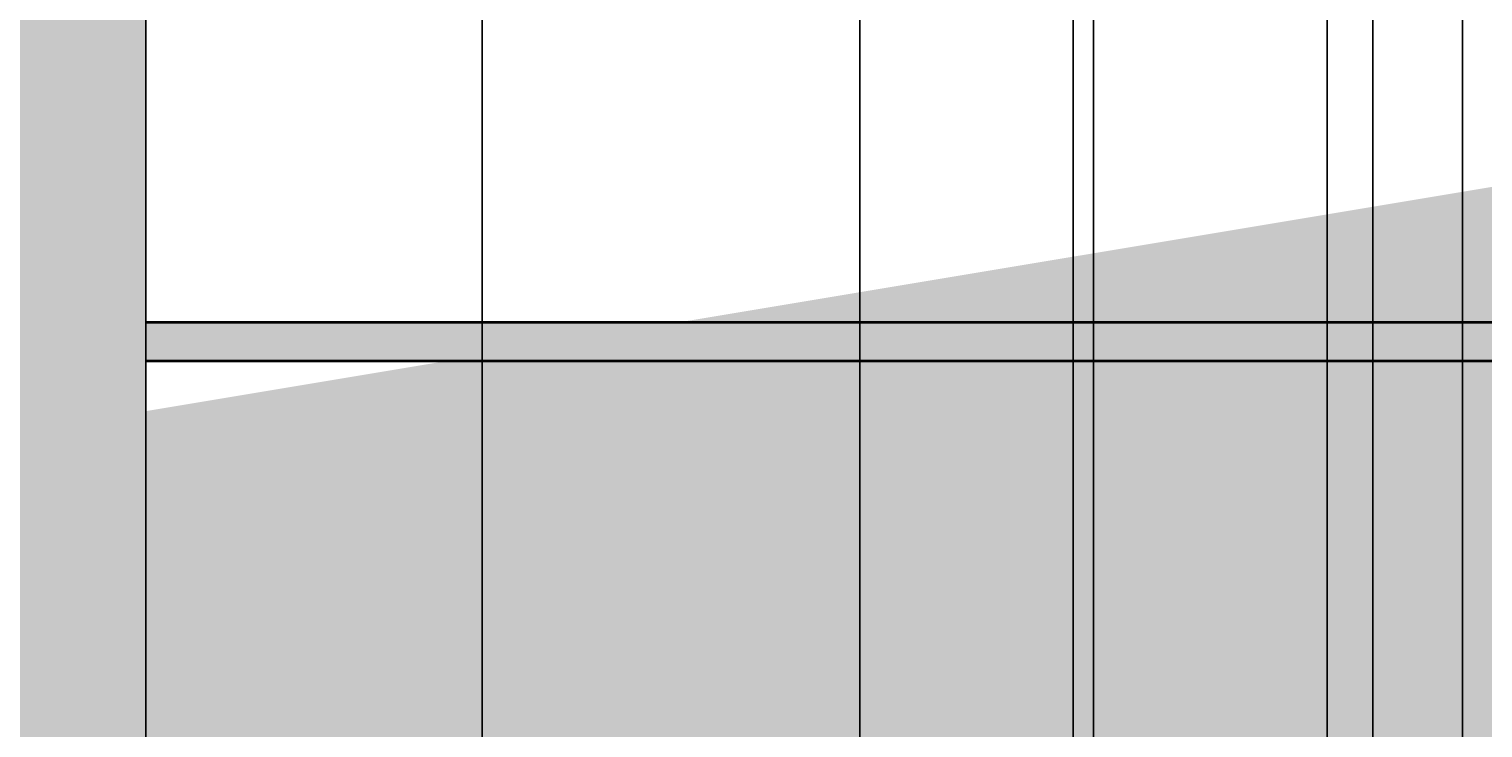
# Model space of a CAD drawing. Units: millimetres. Extents: x -22994 to 29398, y -19990 to 20176.
# Tile 43 of 135: x 99 to 136, y 78 to 96. Entities that reach past the tile are written whole.
import ezdxf

# ---------------------------------------------------------------- set-up
doc = ezdxf.new("R2010")
doc.units = ezdxf.units.MM
doc.header["$MEASUREMENT"] = 0
for name, color, linetype, lineweight in [('M-DIMS', 2, 'Continuous', 18), ('M-EQPM', 7, 'Continuous', 25), ('M-EQPM-PATT', 7, 'Continuous', 18), ('M-PIPE', 7, 'Continuous', 35)]:
    doc.layers.add(name, color=color, linetype=linetype, lineweight=lineweight)
doc.styles.get("Standard").update_dxf_attribs({"font": 'arial.ttf'})
doc.dimstyles.get("Standard").update_dxf_attribs({"dimtxt": 0.18, "dimasz": 10000, "dimexe": 0.18, "dimexo": 0.0625, "dimgap": 0.09, "dimtad": 0, "dimtih": 1, "dimtoh": 1, "dimdec": 0, "dimzin": 0, "dimdsep": 46, "dimtxsty": 'Standard', "dimcen": 0.09, "dimadec": 0, "dimazin": 0, "dimtfac": 1, "dimtdec": 0, "dimtofl": 0, "dimtmove": 0, "dimatfit": 3, "dimfxl": 1, "dimtolj": 1, "dimtzin": 0, "dimlwd": 30, "dimarcsym": 0})

# ---------------------------------------------------------------- blocks, each defined once
blk = doc.blocks.new('*D2')
at = {"layer": 'Defpoints', "color": 0, "transparency": 16777216}
for p in [(6.677, 10.271), (290.852, 10.271), (290.852, -5.079)]:
    blk.add_point(p, dxfattribs=at)
at = {"layer": 'M-DIMS', "color": 0, "lineweight": -2, "transparency": 16777216}
for p, q in [((6.677, 10.209), (6.677, -5.259)), ((290.852, 10.209), (290.852, -5.259))]:
    blk.add_line(p, q, dxfattribs=at)
at = {"layer": 'M-DIMS', "color": 0, "lineweight": 30, "transparency": 16777216}
for p, q in [((-9993.323, -5.079), (-19993.323, -5.079)), ((10290.852, -5.079), (20290.852, -5.079))]:
    blk.add_line(p, q, dxfattribs=at)
at = {"layer": 'M-DIMS', "color": 0, "transparency": 16777216}
for points in [[(-9993.323, 1661.588), (-9993.323, -1671.745), (6.677, -5.079)], [(10290.852, 1661.588), (10290.852, -1671.745), (290.852, -5.079)]]:
    blk.add_solid(points, dxfattribs=at)
at = {"layer": 'M-DIMS', "color": 0, "transparency": 16777216, "insert": (148.765, -5.079), "char_height": 0.18, "attachment_point": 5}
blk.add_mtext('\\A1;284.2', dxfattribs=at)
blk = doc.blocks.new('*D3')
at = {"layer": 'Defpoints', "color": 0, "transparency": 16777216}
for p in [(110.265, 204.165), (110.265, 176.366), (95.833, 127.967)]:
    blk.add_point(p, dxfattribs=at)
at = {"layer": 'M-DIMS', "color": 0, "lineweight": -2, "transparency": 16777216}
for p, q in [((95.833, 128.03), (95.833, 204.345)), ((110.265, 176.429), (110.265, 204.345))]:
    blk.add_line(p, q, dxfattribs=at)
at = {"layer": 'M-DIMS', "color": 0, "lineweight": 30, "transparency": 16777216}
for p, q in [((-9904.167, 204.165), (-19904.167, 204.165)), ((10110.265, 204.165), (20110.265, 204.165))]:
    blk.add_line(p, q, dxfattribs=at)
at = {"layer": 'M-DIMS', "color": 0, "transparency": 16777216}
for points in [[(-9904.167, 1870.832), (-9904.167, -1462.501), (95.833, 204.165)], [(10110.265, 1870.832), (10110.265, -1462.501), (110.265, 204.165)]]:
    blk.add_solid(points, dxfattribs=at)
at = {"layer": 'M-DIMS', "color": 0, "transparency": 16777216, "insert": (103.049, 204.165), "char_height": 0.18, "attachment_point": 5}
blk.add_mtext('\\A1;14.432', dxfattribs=at)
blk = doc.blocks.new('*D4')
at = {"layer": 'Defpoints', "color": 0, "transparency": 16777216}
for p in [(116.265, 204.165), (110.265, 176.366), (116.265, 176.366)]:
    blk.add_point(p, dxfattribs=at)
at = {"layer": 'M-DIMS', "color": 0, "lineweight": -2, "transparency": 16777216}
for p, q in [((110.265, 176.429), (110.265, 204.345)), ((116.265, 176.429), (116.265, 204.345))]:
    blk.add_line(p, q, dxfattribs=at)
at = {"layer": 'M-DIMS', "color": 0, "lineweight": 30, "transparency": 16777216}
for p, q in [((-9889.735, 204.165), (-19889.735, 204.165)), ((10116.265, 204.165), (20116.265, 204.165))]:
    blk.add_line(p, q, dxfattribs=at)
at = {"layer": 'M-DIMS', "color": 0, "transparency": 16777216}
for points in [[(-9889.735, 1870.832), (-9889.735, -1462.501), (110.265, 204.165)], [(10116.265, 1870.832), (10116.265, -1462.501), (116.265, 204.165)]]:
    blk.add_solid(points, dxfattribs=at)
at = {"layer": 'M-DIMS', "color": 0, "transparency": 16777216, "insert": (113.265, 204.165), "char_height": 0.18, "attachment_point": 5}
blk.add_mtext('\\A1;6', dxfattribs=at)
blk = doc.blocks.new('*D5')
at = {"layer": 'Defpoints', "color": 0, "transparency": 16777216}
for p in [(181.265, 204.165), (116.265, 176.366), (181.265, 176.366)]:
    blk.add_point(p, dxfattribs=at)
at = {"layer": 'M-DIMS', "color": 0, "lineweight": -2, "transparency": 16777216}
for p, q in [((116.265, 176.429), (116.265, 204.345)), ((181.265, 176.429), (181.265, 204.345))]:
    blk.add_line(p, q, dxfattribs=at)
at = {"layer": 'M-DIMS', "color": 0, "lineweight": 30, "transparency": 16777216}
for p, q in [((-9883.735, 204.165), (-19883.735, 204.165)), ((10181.265, 204.165), (20181.265, 204.165))]:
    blk.add_line(p, q, dxfattribs=at)
at = {"layer": 'M-DIMS', "color": 0, "transparency": 16777216}
for points in [[(-9883.735, 1870.832), (-9883.735, -1462.501), (116.265, 204.165)], [(10181.265, 1870.832), (10181.265, -1462.501), (181.265, 204.165)]]:
    blk.add_solid(points, dxfattribs=at)
at = {"layer": 'M-DIMS', "color": 0, "transparency": 16777216, "insert": (148.765, 204.165), "char_height": 0.18, "attachment_point": 5}
blk.add_mtext('\\A1;65', dxfattribs=at)
blk = doc.blocks.new('*D6')
at = {"layer": 'Defpoints', "color": 0, "transparency": 16777216}
for p in [(187.265, 204.165), (181.265, 176.366), (187.265, 176.366)]:
    blk.add_point(p, dxfattribs=at)
at = {"layer": 'M-DIMS', "color": 0, "lineweight": -2, "transparency": 16777216}
for p, q in [((181.265, 176.429), (181.265, 204.345)), ((187.265, 176.429), (187.265, 204.345))]:
    blk.add_line(p, q, dxfattribs=at)
at = {"layer": 'M-DIMS', "color": 0, "lineweight": 30, "transparency": 16777216}
for p, q in [((-9818.735, 204.165), (-19818.735, 204.165)), ((10187.265, 204.165), (20187.265, 204.165))]:
    blk.add_line(p, q, dxfattribs=at)
at = {"layer": 'M-DIMS', "color": 0, "transparency": 16777216}
for points in [[(-9818.735, 1870.832), (-9818.735, -1462.501), (181.265, 204.165)], [(10187.265, 1870.832), (10187.265, -1462.501), (187.265, 204.165)]]:
    blk.add_solid(points, dxfattribs=at)
at = {"layer": 'M-DIMS', "color": 0, "transparency": 16777216, "insert": (184.265, 204.165), "char_height": 0.18, "attachment_point": 5}
blk.add_mtext('\\A1;6', dxfattribs=at)
blk = doc.blocks.new('*D7')
at = {"layer": 'Defpoints', "color": 0, "transparency": 16777216}
for p in [(201.697, 204.165), (187.265, 176.366), (201.697, 127.967)]:
    blk.add_point(p, dxfattribs=at)
at = {"layer": 'M-DIMS', "color": 0, "lineweight": -2, "transparency": 16777216}
for p, q in [((187.265, 176.429), (187.265, 204.345)), ((201.697, 128.03), (201.697, 204.345))]:
    blk.add_line(p, q, dxfattribs=at)
at = {"layer": 'M-DIMS', "color": 0, "lineweight": 30, "transparency": 16777216}
for p, q in [((-9812.735, 204.165), (-19812.735, 204.165)), ((10201.697, 204.165), (20201.697, 204.165))]:
    blk.add_line(p, q, dxfattribs=at)
at = {"layer": 'M-DIMS', "color": 0, "transparency": 16777216}
for points in [[(-9812.735, 1870.832), (-9812.735, -1462.501), (187.265, 204.165)], [(10201.697, 1870.832), (10201.697, -1462.501), (201.697, 204.165)]]:
    blk.add_solid(points, dxfattribs=at)
at = {"layer": 'M-DIMS', "color": 0, "transparency": 16777216, "insert": (194.481, 204.165), "char_height": 0.18, "attachment_point": 5}
blk.add_mtext('\\A1;14.432', dxfattribs=at)
blk = doc.blocks.new('*D8')
at = {"layer": 'Defpoints', "color": 0, "transparency": 16777216}
for p in [(227.648, 204.165), (227.648, 146.73), (201.697, 127.967)]:
    blk.add_point(p, dxfattribs=at)
at = {"layer": 'M-DIMS', "color": 0, "lineweight": -2, "transparency": 16777216}
for p, q in [((201.697, 128.03), (201.697, 204.345)), ((227.648, 146.792), (227.648, 204.345))]:
    blk.add_line(p, q, dxfattribs=at)
at = {"layer": 'M-DIMS', "color": 0, "lineweight": 30, "transparency": 16777216}
for p, q in [((-9798.303, 204.165), (-19798.303, 204.165)), ((10227.648, 204.165), (20227.648, 204.165))]:
    blk.add_line(p, q, dxfattribs=at)
at = {"layer": 'M-DIMS', "color": 0, "transparency": 16777216}
for points in [[(-9798.303, 1870.832), (-9798.303, -1462.501), (201.697, 204.165)], [(10227.648, 1870.832), (10227.648, -1462.501), (227.648, 204.165)]]:
    blk.add_solid(points, dxfattribs=at)
at = {"layer": 'M-DIMS', "color": 0, "transparency": 16777216, "insert": (214.673, 204.165), "char_height": 0.18, "attachment_point": 5}
blk.add_mtext('\\A1;25.95', dxfattribs=at)
blk = doc.blocks.new('*D9')
at = {"layer": 'Defpoints', "color": 0, "transparency": 16777216}
for p in [(187.265, 176.366), (306.202, 176.366), (290.852, 10.271)]:
    blk.add_point(p, dxfattribs=at)
at = {"layer": 'M-DIMS', "color": 0, "lineweight": 30, "transparency": 16777216}
for p, q in [((306.202, 10176.366), (306.202, 20176.366)), ((306.202, -9989.729), (306.202, -19989.729))]:
    blk.add_line(p, q, dxfattribs=at)
at = {"layer": 'M-DIMS', "color": 0, "lineweight": -2, "transparency": 16777216}
for p, q in [((187.327, 176.366), (306.382, 176.366)), ((290.915, 10.271), (306.382, 10.271))]:
    blk.add_line(p, q, dxfattribs=at)
at = {"layer": 'M-DIMS', "color": 0, "transparency": 16777216}
for points in [[(-1360.465, 10176.366), (1972.869, 10176.366), (306.202, 176.366)], [(-1360.465, -9989.729), (1972.869, -9989.729), (306.202, 10.271)]]:
    blk.add_solid(points, dxfattribs=at)
at = {"layer": 'M-DIMS', "color": 0, "transparency": 16777216, "insert": (306.202, 93.319), "char_height": 0.18, "attachment_point": 5}
blk.add_mtext('\\A1;166.1', dxfattribs=at)
blk = doc.blocks.new('*D10')
at = {"layer": 'Defpoints', "color": 0, "transparency": 16777216}
for p in [(125.65, 136.071), (133.346, 136.071), (133.346, -5.079)]:
    blk.add_point(p, dxfattribs=at)
at = {"layer": 'M-DIMS', "color": 0, "lineweight": -2, "transparency": 16777216}
for p, q in [((125.65, 136.009), (125.65, -5.259)), ((133.346, 136.009), (133.346, -5.259))]:
    blk.add_line(p, q, dxfattribs=at)
at = {"layer": 'M-DIMS', "color": 0, "lineweight": 30, "transparency": 16777216}
for p, q in [((-9874.35, -5.079), (-19874.35, -5.079)), ((10133.346, -5.079), (20133.346, -5.079))]:
    blk.add_line(p, q, dxfattribs=at)
at = {"layer": 'M-DIMS', "color": 0, "transparency": 16777216}
for points in [[(-9874.35, 1661.588), (-9874.35, -1671.745), (125.65, -5.079)], [(10133.346, 1661.588), (10133.346, -1671.745), (133.346, -5.079)]]:
    blk.add_solid(points, dxfattribs=at)
at = {"layer": 'M-DIMS', "color": 0, "transparency": 16777216, "insert": (129.498, -5.079), "char_height": 0.18, "attachment_point": 5}
blk.add_mtext('\\A1;7.696', dxfattribs=at)
blk = doc.blocks.new('*D11')
at = {"layer": 'Defpoints', "color": 0, "transparency": 16777216}
for p in [(133.346, 136.071), (135.65, 136.071), (135.65, -5.079)]:
    blk.add_point(p, dxfattribs=at)
at = {"layer": 'M-DIMS', "color": 0, "lineweight": -2, "transparency": 16777216}
for p, q in [((133.346, 136.009), (133.346, -5.259)), ((135.65, 136.009), (135.65, -5.259))]:
    blk.add_line(p, q, dxfattribs=at)
at = {"layer": 'M-DIMS', "color": 0, "lineweight": 30, "transparency": 16777216}
for p, q in [((-9866.654, -5.079), (-19866.654, -5.079)), ((10135.65, -5.079), (20135.65, -5.079))]:
    blk.add_line(p, q, dxfattribs=at)
at = {"layer": 'M-DIMS', "color": 0, "transparency": 16777216}
for points in [[(-9866.654, 1661.588), (-9866.654, -1671.745), (133.346, -5.079)], [(10135.65, 1661.588), (10135.65, -1671.745), (135.65, -5.079)]]:
    blk.add_solid(points, dxfattribs=at)
at = {"layer": 'M-DIMS', "color": 0, "transparency": 16777216, "insert": (134.498, -5.079), "char_height": 0.18, "attachment_point": 5}
blk.add_mtext('\\A1;2.304', dxfattribs=at)
blk = doc.blocks.new('*D12')
at = {"layer": 'Defpoints', "color": 0, "transparency": 16777216}
for p in [(135.65, 136.071), (145.65, 136.071), (145.65, -5.079)]:
    blk.add_point(p, dxfattribs=at)
at = {"layer": 'M-DIMS', "color": 0, "lineweight": -2, "transparency": 16777216}
for p, q in [((135.65, 136.009), (135.65, -5.259)), ((145.65, 136.009), (145.65, -5.259))]:
    blk.add_line(p, q, dxfattribs=at)
at = {"layer": 'M-DIMS', "color": 0, "lineweight": 30, "transparency": 16777216}
for p, q in [((-9864.35, -5.079), (-19864.35, -5.079)), ((10145.65, -5.079), (20145.65, -5.079))]:
    blk.add_line(p, q, dxfattribs=at)
at = {"layer": 'M-DIMS', "color": 0, "transparency": 16777216}
for points in [[(-9864.35, 1661.588), (-9864.35, -1671.745), (135.65, -5.079)], [(10145.65, 1661.588), (10145.65, -1671.745), (145.65, -5.079)]]:
    blk.add_solid(points, dxfattribs=at)
at = {"layer": 'M-DIMS', "color": 0, "transparency": 16777216, "insert": (140.65, -5.079), "char_height": 0.18, "attachment_point": 5}
blk.add_mtext('\\A1;10', dxfattribs=at)
blk = doc.blocks.new('*D13')
at = {"layer": 'Defpoints', "color": 0, "transparency": 16777216}
for p in [(145.65, 136.071), (155.65, 136.071), (155.65, -5.079)]:
    blk.add_point(p, dxfattribs=at)
at = {"layer": 'M-DIMS', "color": 0, "lineweight": -2, "transparency": 16777216}
for p, q in [((145.65, 136.009), (145.65, -5.259)), ((155.65, 136.009), (155.65, -5.259))]:
    blk.add_line(p, q, dxfattribs=at)
at = {"layer": 'M-DIMS', "color": 0, "lineweight": 30, "transparency": 16777216}
for p, q in [((-9854.35, -5.079), (-19854.35, -5.079)), ((10155.65, -5.079), (20155.65, -5.079))]:
    blk.add_line(p, q, dxfattribs=at)
at = {"layer": 'M-DIMS', "color": 0, "transparency": 16777216}
for points in [[(-9854.35, 1661.588), (-9854.35, -1671.745), (145.65, -5.079)], [(10155.65, 1661.588), (10155.65, -1671.745), (155.65, -5.079)]]:
    blk.add_solid(points, dxfattribs=at)
at = {"layer": 'M-DIMS', "color": 0, "transparency": 16777216, "insert": (150.65, -5.079), "char_height": 0.18, "attachment_point": 5}
blk.add_mtext('\\A1;10', dxfattribs=at)
blk = doc.blocks.new('*D14')
at = {"layer": 'Defpoints', "color": 0, "transparency": 16777216}
for p in [(155.65, 136.071), (165.65, 136.071), (165.65, -5.079)]:
    blk.add_point(p, dxfattribs=at)
at = {"layer": 'M-DIMS', "color": 0, "lineweight": -2, "transparency": 16777216}
for p, q in [((155.65, 136.009), (155.65, -5.259)), ((165.65, 136.009), (165.65, -5.259))]:
    blk.add_line(p, q, dxfattribs=at)
at = {"layer": 'M-DIMS', "color": 0, "lineweight": 30, "transparency": 16777216}
for p, q in [((-9844.35, -5.079), (-19844.35, -5.079)), ((10165.65, -5.079), (20165.65, -5.079))]:
    blk.add_line(p, q, dxfattribs=at)
at = {"layer": 'M-DIMS', "color": 0, "transparency": 16777216}
for points in [[(-9844.35, 1661.588), (-9844.35, -1671.745), (155.65, -5.079)], [(10165.65, 1661.588), (10165.65, -1671.745), (165.65, -5.079)]]:
    blk.add_solid(points, dxfattribs=at)
at = {"layer": 'M-DIMS', "color": 0, "transparency": 16777216, "insert": (160.65, -5.079), "char_height": 0.18, "attachment_point": 5}
blk.add_mtext('\\A1;10', dxfattribs=at)
blk = doc.blocks.new('*D15')
at = {"layer": 'Defpoints', "color": 0, "transparency": 16777216}
for p in [(173.346, 154.788), (173.346, 136.071), (306.202, 136.071)]:
    blk.add_point(p, dxfattribs=at)
at = {"layer": 'M-DIMS', "color": 0, "lineweight": 30, "transparency": 16777216}
for p, q in [((306.202, 10154.788), (306.202, 20154.788)), ((306.202, -9863.929), (306.202, -19863.929))]:
    blk.add_line(p, q, dxfattribs=at)
at = {"layer": 'M-DIMS', "color": 0, "lineweight": -2, "transparency": 16777216}
for p, q in [((173.408, 154.788), (306.382, 154.788)), ((173.408, 136.071), (306.382, 136.071))]:
    blk.add_line(p, q, dxfattribs=at)
at = {"layer": 'M-DIMS', "color": 0, "transparency": 16777216}
for points in [[(-1360.465, 10154.788), (1972.869, 10154.788), (306.202, 154.788)], [(-1360.465, -9863.929), (1972.869, -9863.929), (306.202, 136.071)]]:
    blk.add_solid(points, dxfattribs=at)
at = {"layer": 'M-DIMS', "color": 0, "transparency": 16777216, "insert": (306.202, 145.43), "char_height": 0.18, "attachment_point": 5}
blk.add_mtext('\\A1;18.717', dxfattribs=at)
blk = doc.blocks.new('*D16')
at = {"layer": 'Defpoints', "color": 0, "transparency": 16777216}
for p in [(120.17, 204.165), (110.466, 48.035), (120.17, 48.035)]:
    blk.add_point(p, dxfattribs=at)
at = {"layer": 'M-DIMS', "color": 0, "lineweight": -2, "transparency": 16777216}
for p, q in [((110.466, 48.097), (110.466, 204.345)), ((120.17, 48.097), (120.17, 204.345))]:
    blk.add_line(p, q, dxfattribs=at)
at = {"layer": 'M-DIMS', "color": 0, "lineweight": 30, "transparency": 16777216}
for p, q in [((-9889.534, 204.165), (-19889.534, 204.165)), ((10120.17, 204.165), (20120.17, 204.165))]:
    blk.add_line(p, q, dxfattribs=at)
at = {"layer": 'M-DIMS', "color": 0, "transparency": 16777216}
for points in [[(-9889.534, 1870.832), (-9889.534, -1462.501), (110.466, 204.165)], [(10120.17, 1870.832), (10120.17, -1462.501), (120.17, 204.165)]]:
    blk.add_solid(points, dxfattribs=at)
at = {"layer": 'M-DIMS', "color": 0, "transparency": 16777216, "insert": (115.318, 204.165), "char_height": 0.18, "attachment_point": 5}
blk.add_mtext('\\A1;9.704', dxfattribs=at)
blk = doc.blocks.new('*D17')
at = {"layer": 'Defpoints', "color": 0, "transparency": 16777216}
for p in [(126.17, 204.165), (120.17, 48.035), (126.17, 48.035)]:
    blk.add_point(p, dxfattribs=at)
at = {"layer": 'M-DIMS', "color": 0, "lineweight": -2, "transparency": 16777216}
for p, q in [((120.17, 48.097), (120.17, 204.345)), ((126.17, 48.097), (126.17, 204.345))]:
    blk.add_line(p, q, dxfattribs=at)
at = {"layer": 'M-DIMS', "color": 0, "lineweight": 30, "transparency": 16777216}
for p, q in [((-9879.83, 204.165), (-19879.83, 204.165)), ((10126.17, 204.165), (20126.17, 204.165))]:
    blk.add_line(p, q, dxfattribs=at)
at = {"layer": 'M-DIMS', "color": 0, "transparency": 16777216}
for points in [[(-9879.83, 1870.832), (-9879.83, -1462.501), (120.17, 204.165)], [(10126.17, 1870.832), (10126.17, -1462.501), (126.17, 204.165)]]:
    blk.add_solid(points, dxfattribs=at)
at = {"layer": 'M-DIMS', "color": 0, "transparency": 16777216, "insert": (123.17, 204.165), "char_height": 0.18, "attachment_point": 5}
blk.add_mtext('\\A1;6', dxfattribs=at)
blk = doc.blocks.new('*D18')
at = {"layer": 'Defpoints', "color": 0, "transparency": 16777216}
for p in [(132.17, 204.165), (126.17, 48.035), (132.17, 48.035)]:
    blk.add_point(p, dxfattribs=at)
at = {"layer": 'M-DIMS', "color": 0, "lineweight": -2, "transparency": 16777216}
for p, q in [((126.17, 48.097), (126.17, 204.345)), ((132.17, 48.097), (132.17, 204.345))]:
    blk.add_line(p, q, dxfattribs=at)
at = {"layer": 'M-DIMS', "color": 0, "lineweight": 30, "transparency": 16777216}
for p, q in [((-9873.83, 204.165), (-19873.83, 204.165)), ((10132.17, 204.165), (20132.17, 204.165))]:
    blk.add_line(p, q, dxfattribs=at)
at = {"layer": 'M-DIMS', "color": 0, "transparency": 16777216}
for points in [[(-9873.83, 1870.832), (-9873.83, -1462.501), (126.17, 204.165)], [(10132.17, 1870.832), (10132.17, -1462.501), (132.17, 204.165)]]:
    blk.add_solid(points, dxfattribs=at)
at = {"layer": 'M-DIMS', "color": 0, "transparency": 16777216, "insert": (129.17, 204.165), "char_height": 0.18, "attachment_point": 5}
blk.add_mtext('\\A1;6', dxfattribs=at)
blk = doc.blocks.new('*D19')
at = {"layer": 'Defpoints', "color": 0, "transparency": 16777216}
for p in [(138.17, 204.165), (132.17, 48.035), (138.17, 48.035)]:
    blk.add_point(p, dxfattribs=at)
at = {"layer": 'M-DIMS', "color": 0, "lineweight": -2, "transparency": 16777216}
for p, q in [((132.17, 48.097), (132.17, 204.345)), ((138.17, 48.097), (138.17, 204.345))]:
    blk.add_line(p, q, dxfattribs=at)
at = {"layer": 'M-DIMS', "color": 0, "lineweight": 30, "transparency": 16777216}
for p, q in [((-9867.83, 204.165), (-19867.83, 204.165)), ((10138.17, 204.165), (20138.17, 204.165))]:
    blk.add_line(p, q, dxfattribs=at)
at = {"layer": 'M-DIMS', "color": 0, "transparency": 16777216}
for points in [[(-9867.83, 1870.832), (-9867.83, -1462.501), (132.17, 204.165)], [(10138.17, 1870.832), (10138.17, -1462.501), (138.17, 204.165)]]:
    blk.add_solid(points, dxfattribs=at)
at = {"layer": 'M-DIMS', "color": 0, "transparency": 16777216, "insert": (135.17, 204.165), "char_height": 0.18, "attachment_point": 5}
blk.add_mtext('\\A1;6', dxfattribs=at)
blk = doc.blocks.new('*D20')
at = {"layer": 'Defpoints', "color": 0, "transparency": 16777216}
for p in [(144.17, 204.165), (138.17, 48.035), (144.17, 48.035)]:
    blk.add_point(p, dxfattribs=at)
at = {"layer": 'M-DIMS', "color": 0, "lineweight": -2, "transparency": 16777216}
for p, q in [((138.17, 48.097), (138.17, 204.345)), ((144.17, 48.097), (144.17, 204.345))]:
    blk.add_line(p, q, dxfattribs=at)
at = {"layer": 'M-DIMS', "color": 0, "lineweight": 30, "transparency": 16777216}
for p, q in [((-9861.83, 204.165), (-19861.83, 204.165)), ((10144.17, 204.165), (20144.17, 204.165))]:
    blk.add_line(p, q, dxfattribs=at)
at = {"layer": 'M-DIMS', "color": 0, "transparency": 16777216}
for points in [[(-9861.83, 1870.832), (-9861.83, -1462.501), (138.17, 204.165)], [(10144.17, 1870.832), (10144.17, -1462.501), (144.17, 204.165)]]:
    blk.add_solid(points, dxfattribs=at)
at = {"layer": 'M-DIMS', "color": 0, "transparency": 16777216, "insert": (141.17, 204.165), "char_height": 0.18, "attachment_point": 5}
blk.add_mtext('\\A1;6', dxfattribs=at)
blk = doc.blocks.new('*D21')
at = {"layer": 'Defpoints', "color": 0, "transparency": 16777216}
for p in [(149.116, 204.165), (144.17, 48.035), (149.116, 48.035)]:
    blk.add_point(p, dxfattribs=at)
at = {"layer": 'M-DIMS', "color": 0, "lineweight": -2, "transparency": 16777216}
for p, q in [((144.17, 48.097), (144.17, 204.345)), ((149.116, 48.097), (149.116, 204.345))]:
    blk.add_line(p, q, dxfattribs=at)
at = {"layer": 'M-DIMS', "color": 0, "lineweight": 30, "transparency": 16777216}
for p, q in [((-9855.83, 204.165), (-19855.83, 204.165)), ((10149.116, 204.165), (20149.116, 204.165))]:
    blk.add_line(p, q, dxfattribs=at)
at = {"layer": 'M-DIMS', "color": 0, "transparency": 16777216}
for points in [[(-9855.83, 1870.832), (-9855.83, -1462.501), (144.17, 204.165)], [(10149.116, 1870.832), (10149.116, -1462.501), (149.116, 204.165)]]:
    blk.add_solid(points, dxfattribs=at)
at = {"layer": 'M-DIMS', "color": 0, "transparency": 16777216, "insert": (146.643, 204.165), "char_height": 0.18, "attachment_point": 5}
blk.add_mtext('\\A1;4.945', dxfattribs=at)
blk = doc.blocks.new('*D22')
at = {"layer": 'Defpoints', "color": 0, "transparency": 16777216}
for p in [(149.116, 30.99), (155.116, 30.99), (155.116, -5.079)]:
    blk.add_point(p, dxfattribs=at)
at = {"layer": 'M-DIMS', "color": 0, "lineweight": -2, "transparency": 16777216}
for p, q in [((149.116, 30.927), (149.116, -5.259)), ((155.116, 30.927), (155.116, -5.259))]:
    blk.add_line(p, q, dxfattribs=at)
at = {"layer": 'M-DIMS', "color": 0, "lineweight": 30, "transparency": 16777216}
for p, q in [((-9850.884, -5.079), (-19850.884, -5.079)), ((10155.116, -5.079), (20155.116, -5.079))]:
    blk.add_line(p, q, dxfattribs=at)
at = {"layer": 'M-DIMS', "color": 0, "transparency": 16777216}
for points in [[(-9850.884, 1661.588), (-9850.884, -1671.745), (149.116, -5.079)], [(10155.116, 1661.588), (10155.116, -1671.745), (155.116, -5.079)]]:
    blk.add_solid(points, dxfattribs=at)
at = {"layer": 'M-DIMS', "color": 0, "transparency": 16777216, "insert": (152.116, -5.079), "char_height": 0.18, "attachment_point": 5}
blk.add_mtext('\\A1;6', dxfattribs=at)
blk = doc.blocks.new('*D23')
at = {"layer": 'Defpoints', "color": 0, "transparency": 16777216}
for p in [(155.116, 30.99), (161.116, 30.99), (161.116, -5.079)]:
    blk.add_point(p, dxfattribs=at)
at = {"layer": 'M-DIMS', "color": 0, "lineweight": -2, "transparency": 16777216}
for p, q in [((155.116, 30.927), (155.116, -5.259)), ((161.116, 30.927), (161.116, -5.259))]:
    blk.add_line(p, q, dxfattribs=at)
at = {"layer": 'M-DIMS', "color": 0, "lineweight": 30, "transparency": 16777216}
for p, q in [((-9844.884, -5.079), (-19844.884, -5.079)), ((10161.116, -5.079), (20161.116, -5.079))]:
    blk.add_line(p, q, dxfattribs=at)
at = {"layer": 'M-DIMS', "color": 0, "transparency": 16777216}
for points in [[(-9844.884, 1661.588), (-9844.884, -1671.745), (155.116, -5.079)], [(10161.116, 1661.588), (10161.116, -1671.745), (161.116, -5.079)]]:
    blk.add_solid(points, dxfattribs=at)
at = {"layer": 'M-DIMS', "color": 0, "transparency": 16777216, "insert": (158.116, -5.079), "char_height": 0.18, "attachment_point": 5}
blk.add_mtext('\\A1;6', dxfattribs=at)
blk = doc.blocks.new('*D24')
at = {"layer": 'Defpoints', "color": 0, "transparency": 16777216}
for p in [(161.116, 30.99), (166.439, 30.99), (166.439, -5.079)]:
    blk.add_point(p, dxfattribs=at)
at = {"layer": 'M-DIMS', "color": 0, "lineweight": -2, "transparency": 16777216}
for p, q in [((161.116, 30.927), (161.116, -5.259)), ((166.439, 30.927), (166.439, -5.259))]:
    blk.add_line(p, q, dxfattribs=at)
at = {"layer": 'M-DIMS', "color": 0, "lineweight": 30, "transparency": 16777216}
for p, q in [((-9838.884, -5.079), (-19838.884, -5.079)), ((10166.439, -5.079), (20166.439, -5.079))]:
    blk.add_line(p, q, dxfattribs=at)
at = {"layer": 'M-DIMS', "color": 0, "transparency": 16777216}
for points in [[(-9838.884, 1661.588), (-9838.884, -1671.745), (161.116, -5.079)], [(10166.439, 1661.588), (10166.439, -1671.745), (166.439, -5.079)]]:
    blk.add_solid(points, dxfattribs=at)
at = {"layer": 'M-DIMS', "color": 0, "transparency": 16777216, "insert": (163.777, -5.079), "char_height": 0.18, "attachment_point": 5}
blk.add_mtext('\\A1;5.323', dxfattribs=at)
blk = doc.blocks.new('*D25')
at = {"layer": 'Defpoints', "color": 0, "transparency": 16777216}
for p in [(166.439, 30.99), (172.439, 30.99), (172.439, -5.079)]:
    blk.add_point(p, dxfattribs=at)
at = {"layer": 'M-DIMS', "color": 0, "lineweight": -2, "transparency": 16777216}
for p, q in [((166.439, 30.927), (166.439, -5.259)), ((172.439, 30.927), (172.439, -5.259))]:
    blk.add_line(p, q, dxfattribs=at)
at = {"layer": 'M-DIMS', "color": 0, "lineweight": 30, "transparency": 16777216}
for p, q in [((-9833.561, -5.079), (-19833.561, -5.079)), ((10172.439, -5.079), (20172.439, -5.079))]:
    blk.add_line(p, q, dxfattribs=at)
at = {"layer": 'M-DIMS', "color": 0, "transparency": 16777216}
for points in [[(-9833.561, 1661.588), (-9833.561, -1671.745), (166.439, -5.079)], [(10172.439, 1661.588), (10172.439, -1671.745), (172.439, -5.079)]]:
    blk.add_solid(points, dxfattribs=at)
at = {"layer": 'M-DIMS', "color": 0, "transparency": 16777216, "insert": (169.439, -5.079), "char_height": 0.18, "attachment_point": 5}
blk.add_mtext('\\A1;6', dxfattribs=at)
blk = doc.blocks.new('*D26')
at = {"layer": 'Defpoints', "color": 0, "transparency": 16777216}
for p in [(172.439, 30.99), (178.439, 30.99), (178.439, -5.079)]:
    blk.add_point(p, dxfattribs=at)
at = {"layer": 'M-DIMS', "color": 0, "lineweight": -2, "transparency": 16777216}
for p, q in [((172.439, 30.927), (172.439, -5.259)), ((178.439, 30.927), (178.439, -5.259))]:
    blk.add_line(p, q, dxfattribs=at)
at = {"layer": 'M-DIMS', "color": 0, "lineweight": 30, "transparency": 16777216}
for p, q in [((-9827.561, -5.079), (-19827.561, -5.079)), ((10178.439, -5.079), (20178.439, -5.079))]:
    blk.add_line(p, q, dxfattribs=at)
at = {"layer": 'M-DIMS', "color": 0, "transparency": 16777216}
for points in [[(-9827.561, 1661.588), (-9827.561, -1671.745), (172.439, -5.079)], [(10178.439, 1661.588), (10178.439, -1671.745), (178.439, -5.079)]]:
    blk.add_solid(points, dxfattribs=at)
at = {"layer": 'M-DIMS', "color": 0, "transparency": 16777216, "insert": (175.439, -5.079), "char_height": 0.18, "attachment_point": 5}
blk.add_mtext('\\A1;6', dxfattribs=at)
blk = doc.blocks.new('*D27')
at = {"layer": 'Defpoints', "color": 0, "transparency": 16777216}
for p in [(178.439, 30.99), (188.117, 30.99), (188.117, -5.079)]:
    blk.add_point(p, dxfattribs=at)
at = {"layer": 'M-DIMS', "color": 0, "lineweight": -2, "transparency": 16777216}
for p, q in [((178.439, 30.927), (178.439, -5.259)), ((188.117, 30.927), (188.117, -5.259))]:
    blk.add_line(p, q, dxfattribs=at)
at = {"layer": 'M-DIMS', "color": 0, "lineweight": 30, "transparency": 16777216}
for p, q in [((-9821.561, -5.079), (-19821.561, -5.079)), ((10188.117, -5.079), (20188.117, -5.079))]:
    blk.add_line(p, q, dxfattribs=at)
at = {"layer": 'M-DIMS', "color": 0, "transparency": 16777216}
for points in [[(-9821.561, 1661.588), (-9821.561, -1671.745), (178.439, -5.079)], [(10188.117, 1661.588), (10188.117, -1671.745), (188.117, -5.079)]]:
    blk.add_solid(points, dxfattribs=at)
at = {"layer": 'M-DIMS', "color": 0, "transparency": 16777216, "insert": (183.278, -5.079), "char_height": 0.18, "attachment_point": 5}
blk.add_mtext('\\A1;9.679', dxfattribs=at)
blk = doc.blocks.new('*D28')
at = {"layer": 'Defpoints', "color": 0, "transparency": 16777216}
for p in [(188.117, 48.035), (306.202, 48.035), (188.117, 30.99)]:
    blk.add_point(p, dxfattribs=at)
at = {"layer": 'M-DIMS', "color": 0, "lineweight": 30, "transparency": 16777216}
for p, q in [((306.202, 10048.035), (306.202, 20048.035)), ((306.202, -9969.01), (306.202, -19969.01))]:
    blk.add_line(p, q, dxfattribs=at)
at = {"layer": 'M-DIMS', "color": 0, "lineweight": -2, "transparency": 16777216}
for p, q in [((188.18, 48.035), (306.382, 48.035)), ((188.18, 30.99), (306.382, 30.99))]:
    blk.add_line(p, q, dxfattribs=at)
at = {"layer": 'M-DIMS', "color": 0, "transparency": 16777216}
for points in [[(-1360.465, 10048.035), (1972.869, 10048.035), (306.202, 48.035)], [(-1360.465, -9969.01), (1972.869, -9969.01), (306.202, 30.99)]]:
    blk.add_solid(points, dxfattribs=at)
at = {"layer": 'M-DIMS', "color": 0, "transparency": 16777216, "insert": (306.202, 39.512), "char_height": 0.18, "attachment_point": 5}
blk.add_mtext('\\A1;17.045', dxfattribs=at)
blk = doc.blocks.new('*D29')
at = {"layer": 'Defpoints', "color": 0, "transparency": 16777216}
for p in [(36.801, 80.045), (64.03, 80.045)]:
    blk.add_point(p, dxfattribs=at)
at = {"layer": 'M-DIMS', "color": 0, "lineweight": -2, "transparency": 16777216}
for p, q in [((50.325, 80.045), (50.505, 80.045)), ((50.415, 79.955), (50.415, 80.135))]:
    blk.add_line(p, q, dxfattribs=at)
at = {"layer": 'M-DIMS', "color": 0, "lineweight": 30, "transparency": 16777216}
blk.add_line((20064.03, 80.03), (10064.03, 80.038), dxfattribs=at)
at = {"layer": 'M-DIMS', "color": 0, "transparency": 16777216}
blk.add_solid([(10064.031, 1746.704), (10064.028, -1586.629), (64.03, 80.045)], dxfattribs=at)
at = {"layer": 'M-DIMS', "color": 0, "transparency": 16777216, "insert": (20064.521, 80.03), "char_height": 0.18, "attachment_point": 5}
blk.add_mtext('\\A1;∅27.23', dxfattribs=at)
blk = doc.blocks.new('*D36')
at = {"layer": 'Defpoints', "color": 0, "transparency": 16777216}
for p in [(46.39, 31.303), (46.387, 26.593)]:
    blk.add_point(p, dxfattribs=at)
at = {"layer": 'M-DIMS', "color": 0, "lineweight": 30, "transparency": 16777216}
for p, q in [((57.15, 20031.301), (51.77, 10031.302)), ((10057.15, 20031.301), (57.15, 20031.301))]:
    blk.add_line(p, q, dxfattribs=at)
at = {"layer": 'M-DIMS', "color": 0, "lineweight": -2, "transparency": 16777216}
for p, q in [((46.299, 28.948), (46.479, 28.948)), ((46.389, 28.858), (46.389, 29.038))]:
    blk.add_line(p, q, dxfattribs=at)
at = {"layer": 'M-DIMS', "color": 0, "transparency": 16777216}
blk.add_solid([(-1614.896, 10032.199), (1718.436, 10030.405), (46.39, 31.303)], dxfattribs=at)
at = {"layer": 'M-DIMS', "color": 0, "transparency": 16777216, "insert": (10057.554, 20031.301), "char_height": 0.18, "attachment_point": 5}
blk.add_mtext('\\A1;∅4.71', dxfattribs=at)
blk = doc.blocks.new('*D37')
at = {"layer": 'Defpoints', "color": 0, "transparency": 16777216}
for p in [(54.834, 118.615), (59.494, 118.614)]:
    blk.add_point(p, dxfattribs=at)
at = {"layer": 'M-DIMS', "color": 0, "lineweight": -2, "transparency": 16777216}
for p, q in [((57.074, 118.614), (57.254, 118.614)), ((57.164, 118.524), (57.164, 118.704))]:
    blk.add_line(p, q, dxfattribs=at)
at = {"layer": 'M-DIMS', "color": 0, "lineweight": 30, "transparency": 16777216}
blk.add_line((20059.493, 116.253), (10059.494, 117.434), dxfattribs=at)
at = {"layer": 'M-DIMS', "color": 0, "transparency": 16777216}
blk.add_solid([(10059.69, 1784.1), (10059.297, -1549.233), (59.494, 118.614)], dxfattribs=at)
at = {"layer": 'M-DIMS', "color": 0, "transparency": 16777216, "insert": (20059.985, 116.253), "char_height": 0.18, "attachment_point": 5}
blk.add_mtext('\\A1;∅4.659', dxfattribs=at)

msp = doc.modelspace()

# ---------------------------------------------------------------- hatches: boundary and pattern name
at = {"layer": 'M-EQPM-PATT'}
h = msp.add_hatch(color=256, dxfattribs=at)
h.set_gradient(color1=(205, 32, 39), color2=(205, 32, 39), tint=1)
h.paths.add_polyline_path([(116.2647, 150.3662), (116.2647, 170.3662), (116.2647, 176.3662), (110.2647, 176.3662), (110.2647, 152.0276), (95.8327, 127.967), (95.8327, 16.6063), (201.6967, 16.6063), (201.6967, 127.967), (187.2647, 152.0276), (187.2647, 176.3662), (181.2647, 176.3662), (181.2647, 170.3662), (181.2647, 150.3662), (195.6967, 126.3055), (195.6967, 22.6063), (101.8327, 22.6063), (101.8327, 126.3055)])
h.paths.add_polyline_path([(185.2208, 88.6347), (101.8327, 88.6347), (101.8327, 87.6347), (182.8066, 87.6347), (178.7313, 83.5594), (195.6967, 83.5594), (195.6967, 84.5594), (181.1455, 84.5594)], flags=17)
h.paths.add_polyline_path([(95.8327, 88.6347), (60.9779, 88.6347, -0.0228552), (61.7178, 87.6347), (95.8327, 87.6347)])
h.paths.add_polyline_path([(215.6212, 86.5189), (215.6212, 80.5999), (220.5095, 83.5594)])
h.paths.add_polyline_path([(215.6212, 84.5594), (201.6967, 84.5594), (201.6967, 83.5594), (215.6212, 83.5594)])
h.paths.add_polyline_path([(225.3978, 86.5189), (220.5095, 83.5594), (225.3978, 80.5999)])
h.paths.add_polyline_path([(231.6256, 84.5594), (225.3978, 84.5594), (225.3978, 83.5594), (231.6256, 83.5594)])
h = msp.add_hatch(color=256, dxfattribs=at)
h.set_gradient(color1=(19, 155, 72), color2=(88, 186, 72), tint=1, name='CYLINDER')
h.paths.add_polyline_path([(109.4658, 29.9895), (189.1175, 29.9895), (189.1175, 77.6953), (128.1172, 77.6953, 0.4142136), (126.1172, 75.6953), (126.1172, 73.6953, 0.4142136), (128.1172, 71.6953), (178.5136, 71.6953, -0.4142136), (179.5136, 70.6953), (179.5136, 68.6953, -0.4142136), (178.5136, 67.6953), (128.1172, 67.6953, 0.4142136), (126.1172, 65.6953), (126.1172, 63.6953, 0.4142136), (128.1172, 61.6953), (178.5136, 61.6953, -0.4142136), (179.5136, 60.6953), (179.5136, 58.6953, -0.4142136), (178.5136, 57.6953), (109.7466, 57.6953, -0.4142136), (108.7466, 58.6953), (108.7466, 75.5922, 0.4142136), (106.7466, 77.5922), (101.8327, 77.5922), (101.8327, 76.5922), (106.7466, 76.5922, -0.4142136), (107.7466, 75.5922), (107.7466, 58.6953, 0.4142136), (109.7466, 56.6953), (178.5136, 56.6953, 0.4142136), (180.5136, 58.6953), (180.5136, 60.6953, 0.4142136), (178.5136, 62.6953), (128.1172, 62.6953, -0.4142136), (127.1172, 63.6953), (127.1172, 65.6953, -0.4142136), (128.1172, 66.6953), (178.5136, 66.6953, 0.4142136), (180.5136, 68.6953), (180.5136, 70.6953, 0.4142136), (178.5136, 72.6953), (128.1172, 72.6953, -0.4142136), (127.1172, 73.6953), (127.1172, 75.6953, -0.4142136), (128.1172, 76.6953), (188.1175, 76.6953), (188.1175, 49.0349), (110.4658, 49.0349), (110.4658, 51.9576), (101.8327, 51.9576), (101.8327, 50.9576), (109.4658, 50.9576), (109.4658, 48.5349)])
h.paths.add_polyline_path([(110.4658, 48.0349), (188.1175, 48.0349), (188.1175, 30.9895), (110.4658, 30.9895)], flags=16)
h.paths.add_polyline_path([(136.1519, 78.0082), (161.2406, 78.0082), (161.2406, 84.1903), (136.1519, 84.1903)], flags=9)

# ---------------------------------------------------------------- linework, layer by layer
at = {"layer": 'M-EQPM'}
msp.add_lwpolyline([(116.2647, 170.3662), (116.2647, 150.3662), (101.8327, 126.3055), (101.8327, 22.6063), (195.6967, 22.6063), (195.6967, 126.3055), (181.2647, 150.3662), (181.2647, 170.3662)], dxfattribs=at)
at = {"layer": 'M-PIPE'}
for p, q in [((101.8327, 88.6347), (185.2208, 88.6347)), ((101.8327, 87.6347), (182.8066, 87.6347))]:
    msp.add_line(p, q, dxfattribs=at)

# ---------------------------------------------------------------- dimensions: what is measured, and where the dimension line sits
at = {"layer": 'M-DIMS'}
for base, p1, p2, override, picture, middle in [((306.202, 176.3662), (290.852, 10.2713), (187.2647, 176.3662), {"dimdec": 1, "dimlfac": 1, "dimrnd": 0, "dimzin": 0, "dimdsep": 46, "dimlunit": 2}, '*D9', (306.202, 93.3187)), ((306.202, 136.0713), (173.3459, 154.788), (173.3459, 136.0713), {"dimdec": 3, "dimlfac": 1, "dimrnd": 0, "dimzin": 0, "dimdsep": 46, "dimlunit": 2}, '*D15', (306.202, 145.4297)), ((306.202, 48.0349), (188.1175, 30.9895), (188.1175, 48.0349), {"dimdec": 3, "dimlfac": 1, "dimrnd": 0, "dimzin": 0, "dimdsep": 46, "dimlunit": 2}, '*D28', (306.202, 39.5122))]:
    dim = msp.add_linear_dim(base=base, p1=p1, p2=p2, angle=90, dimstyle='Standard', override=override, dxfattribs=at)
    dim.commit()
    dim.dimension.update_dxf_attribs({"geometry": picture, "text_midpoint": middle})
dim = msp.add_diameter_dim_2p(p1=(46.3875, 26.5934), p2=(46.39, 31.3035), dimstyle='Standard', override={"dimdec": 2, "dimlfac": 1, "dimrnd": 0, "dimzin": 0, "dimdsep": 46, "dimlunit": 2}, dxfattribs=at)
dim.commit()
dim.dimension.update_dxf_attribs({"geometry": '*D36', "text_midpoint": (10057.5542, 20031.3006), "dimtype": 163})
for base, p1, p2, override, picture, middle in [((110.2647, 204.1654), (95.8327, 127.967), (110.2647, 176.3662), {"dimdec": 3, "dimlfac": 1, "dimrnd": 0, "dimzin": 0, "dimdsep": 46, "dimlunit": 2}, '*D3', (103.0487, 204.1654)), ((116.2647, 204.1654), (110.2647, 176.3662), (116.2647, 176.3662), {"dimdec": 0, "dimlfac": 1, "dimrnd": 0, "dimzin": 0, "dimdsep": 46, "dimlunit": 2}, '*D4', (113.2647, 204.1654)), ((120.1702, 204.1654), (110.4658, 48.0349), (120.1702, 48.0349), {"dimdec": 3, "dimlfac": 1, "dimrnd": 0, "dimzin": 0, "dimdsep": 46, "dimlunit": 2}, '*D16', (115.318, 204.1654)), ((181.2647, 204.1654), (116.2647, 176.3662), (181.2647, 176.3662), {"dimdec": 0, "dimlfac": 1, "dimrnd": 0, "dimzin": 0, "dimdsep": 46, "dimlunit": 2}, '*D5', (148.7647, 204.1654)), ((126.1702, 204.1654), (120.1702, 48.0349), (126.1702, 48.0349), {"dimdec": 0, "dimlfac": 1, "dimrnd": 0, "dimzin": 0, "dimdsep": 46, "dimlunit": 2}, '*D17', (123.1702, 204.1654)), ((132.1702, 204.1654), (126.1702, 48.0349), (132.1702, 48.0349), {"dimdec": 0, "dimlfac": 1, "dimrnd": 0, "dimzin": 0, "dimdsep": 46, "dimlunit": 2}, '*D18', (129.1702, 204.1654)), ((138.1702, 204.1654), (132.1702, 48.0349), (138.1702, 48.0349), {"dimdec": 0, "dimlfac": 1, "dimrnd": 0, "dimzin": 0, "dimdsep": 46, "dimlunit": 2}, '*D19', (135.1702, 204.1654)), ((144.1702, 204.1654), (138.1702, 48.0349), (144.1702, 48.0349), {"dimdec": 0, "dimlfac": 1, "dimrnd": 0, "dimzin": 0, "dimdsep": 46, "dimlunit": 2}, '*D20', (141.1702, 204.1654)), ((149.11567, 204.16539), (144.17023, 48.03494), (149.11567, 48.03494), {"dimdec": 3, "dimlfac": 1, "dimrnd": 0, "dimzin": 0, "dimdsep": 46, "dimlunit": 2}, '*D21', (146.64295, 204.16539)), ((187.2647, 204.1654), (181.2647, 176.3662), (187.2647, 176.3662), {"dimdec": 0, "dimlfac": 1, "dimrnd": 0, "dimzin": 0, "dimdsep": 46, "dimlunit": 2}, '*D6', (184.2647, 204.1654)), ((201.6967, 204.1654), (187.2647, 176.3662), (201.6967, 127.967), {"dimdec": 3, "dimlfac": 1, "dimrnd": 0, "dimzin": 0, "dimdsep": 46, "dimlunit": 2}, '*D7', (194.4807, 204.1654)), ((227.6485, 204.1654), (201.6967, 127.967), (227.6485, 146.7296), {"dimdec": 2, "dimlfac": 1, "dimrnd": 0, "dimzin": 0, "dimdsep": 46, "dimlunit": 2}, '*D8', (214.6726, 204.1654)), ((290.852, -5.0787), (6.6773, 10.2713), (290.852, 10.2713), {"dimdec": 1, "dimlfac": 1, "dimrnd": 0, "dimzin": 0, "dimdsep": 46, "dimlunit": 2}, '*D2', (148.7647, -5.0787)), ((133.3459, -5.0787), (125.6498, 136.0713), (133.3459, 136.0713), {"dimdec": 3, "dimlfac": 1, "dimrnd": 0, "dimzin": 0, "dimdsep": 46, "dimlunit": 2}, '*D10', (129.4978, -5.0787)), ((135.6498, -5.0787), (133.3459, 136.0713), (135.6498, 136.0713), {"dimdec": 3, "dimlfac": 1, "dimrnd": 0, "dimzin": 0, "dimdsep": 46, "dimlunit": 2}, '*D11', (134.4978, -5.0787)), ((145.6498, -5.0787), (135.6498, 136.0713), (145.6498, 136.0713), {"dimdec": 0, "dimlfac": 1, "dimrnd": 0, "dimzin": 0, "dimdsep": 46, "dimlunit": 2}, '*D12', (140.6498, -5.0787)), ((155.6498, -5.0787), (145.6498, 136.0713), (155.6498, 136.0713), {"dimdec": 0, "dimlfac": 1, "dimrnd": 0, "dimzin": 0, "dimdsep": 46, "dimlunit": 2}, '*D13', (150.6498, -5.0787)), ((155.1157, -5.0787), (149.1157, 30.9895), (155.1157, 30.9895), {"dimdec": 0, "dimlfac": 1, "dimrnd": 0, "dimzin": 0, "dimdsep": 46, "dimlunit": 2}, '*D22', (152.1157, -5.0787)), ((161.1157, -5.0787), (155.1157, 30.9895), (161.1157, 30.9895), {"dimdec": 0, "dimlfac": 1, "dimrnd": 0, "dimzin": 0, "dimdsep": 46, "dimlunit": 2}, '*D23', (158.1157, -5.0787)), ((165.6498, -5.0787), (155.6498, 136.0713), (165.6498, 136.0713), {"dimdec": 0, "dimlfac": 1, "dimrnd": 0, "dimzin": 0, "dimdsep": 46, "dimlunit": 2}, '*D14', (160.6498, -5.0787)), ((166.4387, -5.0787), (161.1157, 30.9895), (166.4387, 30.9895), {"dimdec": 3, "dimlfac": 1, "dimrnd": 0, "dimzin": 0, "dimdsep": 46, "dimlunit": 2}, '*D24', (163.7772, -5.0787)), ((172.4387, -5.0787), (166.4387, 30.9895), (172.4387, 30.9895), {"dimdec": 0, "dimlfac": 1, "dimrnd": 0, "dimzin": 0, "dimdsep": 46, "dimlunit": 2}, '*D25', (169.4387, -5.0787)), ((178.4387, -5.0787), (172.4387, 30.9895), (178.4387, 30.9895), {"dimdec": 0, "dimlfac": 1, "dimrnd": 0, "dimzin": 0, "dimdsep": 46, "dimlunit": 2}, '*D26', (175.4387, -5.0787)), ((188.1175, -5.0787), (178.4387, 30.9895), (188.1175, 30.9895), {"dimdec": 3, "dimlfac": 1, "dimrnd": 0, "dimzin": 0, "dimdsep": 46, "dimlunit": 2}, '*D27', (183.2781, -5.0787))]:
    dim = msp.add_linear_dim(base=base, p1=p1, p2=p2, dimstyle='Standard', override=override, dxfattribs=at)
    dim.commit()
    dim.dimension.update_dxf_attribs({"geometry": picture, "text_midpoint": middle})
for p1, p2, override, picture, middle in [((54.8343, 118.6145), (59.4936, 118.614), {"dimdec": 3, "dimlfac": 1, "dimrnd": 0, "dimzin": 0, "dimdsep": 46, "dimlunit": 2}, '*D37', (20059.4934, 116.2531)), ((36.8006, 80.045), (64.0296, 80.045), {"dimdec": 2, "dimlfac": 1, "dimrnd": 0, "dimzin": 0, "dimdsep": 46, "dimlunit": 2}, '*D29', (20064.0296, 80.0303))]:
    dim = msp.add_diameter_dim_2p(p1=p1, p2=p2, dimstyle='Standard', override=override, dxfattribs=at)
    dim.commit()
    dim.dimension.update_dxf_attribs({"geometry": picture, "text_midpoint": middle})

doc.saveas('drawing.dxf')
